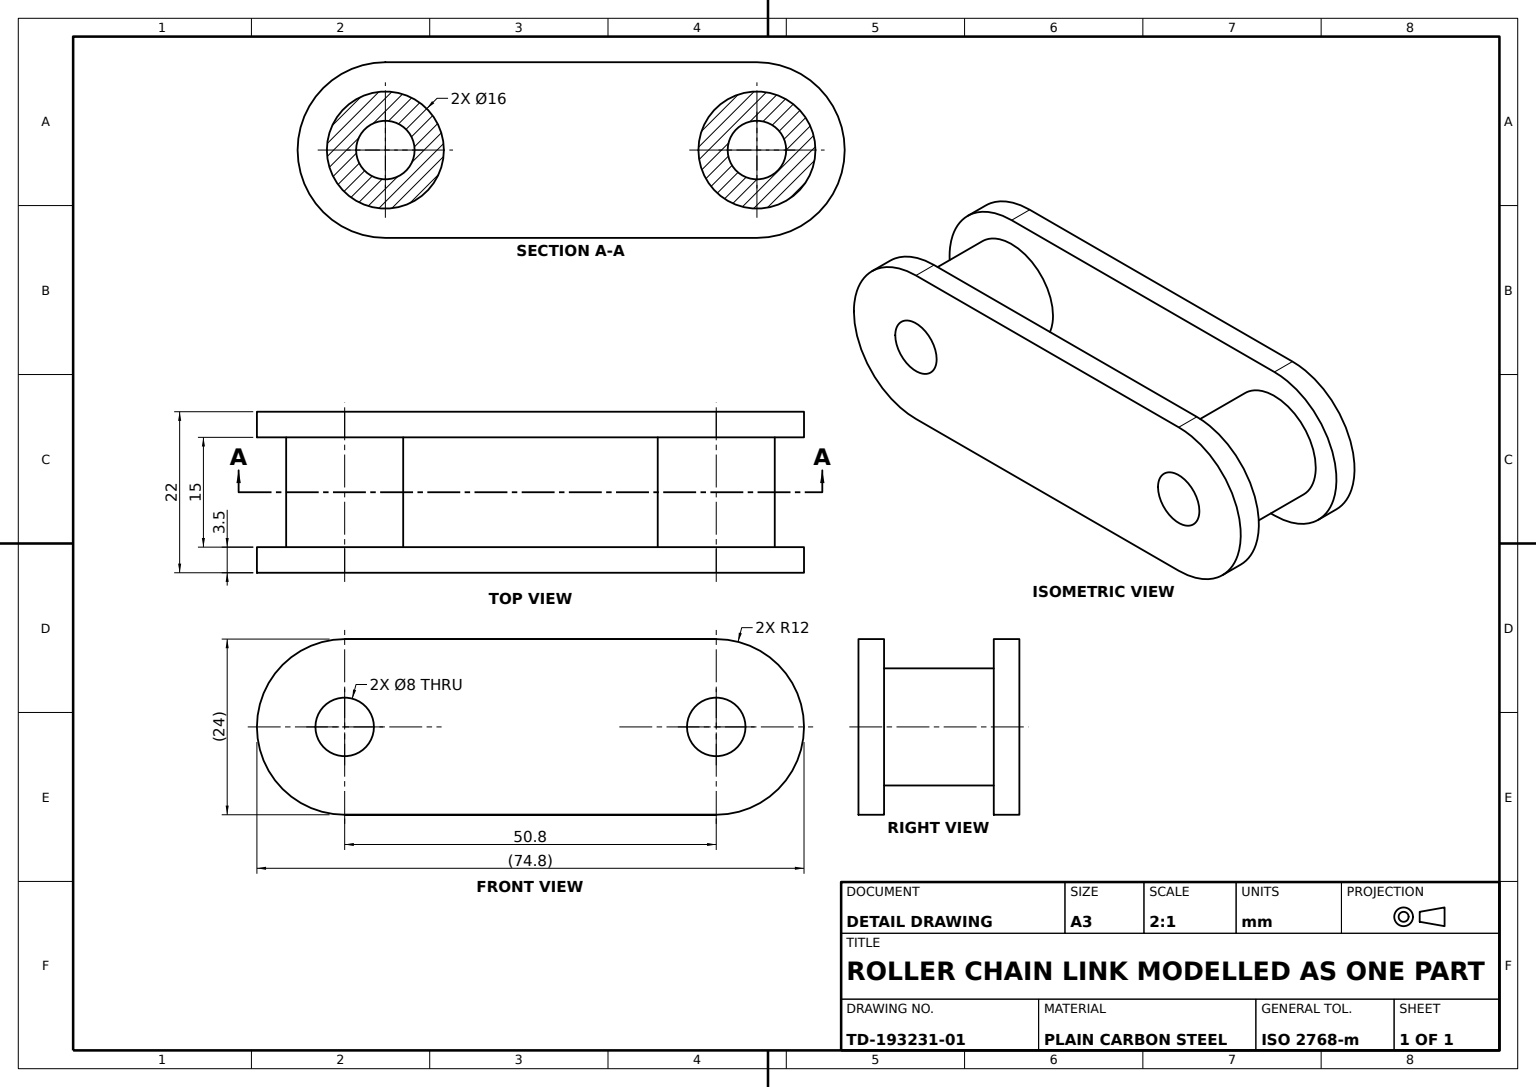
SolidWorks part; units mm, degrees
material "Plain Carbon Steel"
ref_plane "Front Plane" through (0, 0, 0) normal (0, 0, 1) x (1, 0, 0)
ref_plane "Top Plane" through (0, 0, 0) normal (0, 1, 0) x (1, 0, 0)
ref_plane "Right Plane" through (0, 0, 0) normal (1, 0, 0) x (0, 0, -1)
sketch "Rear Plate Profile" plane through (0, 0, 0) normal (0, 0, 1) x (1, 0, 0)
  line L1 (0, 12) -> (50.8, 12)
  line L3 (50.8, -12) -> (0, -12)
  arc A0 (50.8, -12) -> (50.8, 12) centre (50.8, 0) ccw
  arc A1 (0, 12) -> (0, -12) centre (0, 0) ccw
  dimension "D1" = 12
  dimension "D2" = 50.8
extrude "Rear Link Plate" add sketch "Rear Plate Profile" along normal blind 3.5
sketch "Roller Profiles" plane through (0, 0, 3.5) normal (0, 0, 1) x (1, 0, 0)
  circle A0 centre (0, 0) radius 8
  circle A1 centre (50.8, 0) radius 8
  dimension "D1" = 16
  dimension "D2" = 16
  dimension "D3" = 16
extrude "Rollers 2xØ16" add sketch "Roller Profiles" along normal blind 15
sketch "Front Plate Profile" plane through (0, 0, 18.5) normal (0, 0, 1) x (1, 0, 0)
  line L0 (0, 12) -> (50.8, 12)
  line L2 (50.8, -12) -> (0, -12)
  arc A0 (0, 12) -> (0, -12) centre (0, 0) ccw
  arc A1 (50.8, -12) -> (50.8, 12) centre (50.8, 0) ccw
extrude "Front Link Plate" add sketch "Front Plate Profile" along normal blind 3.5
sketch "Pin Bore Profiles" plane through (0, 0, 22) normal (0, 0, 1) x (1, 0, 0)
  circle A0 centre (0, 0) radius 4
  circle A1 centre (50.8, 0) radius 4
  dimension "D1" = 8
  dimension "D2" = 8
  dimension "D3" = 8
extrude "Pin Bores 2xØ8" cut sketch "Pin Bore Profiles" against normal blind 22
